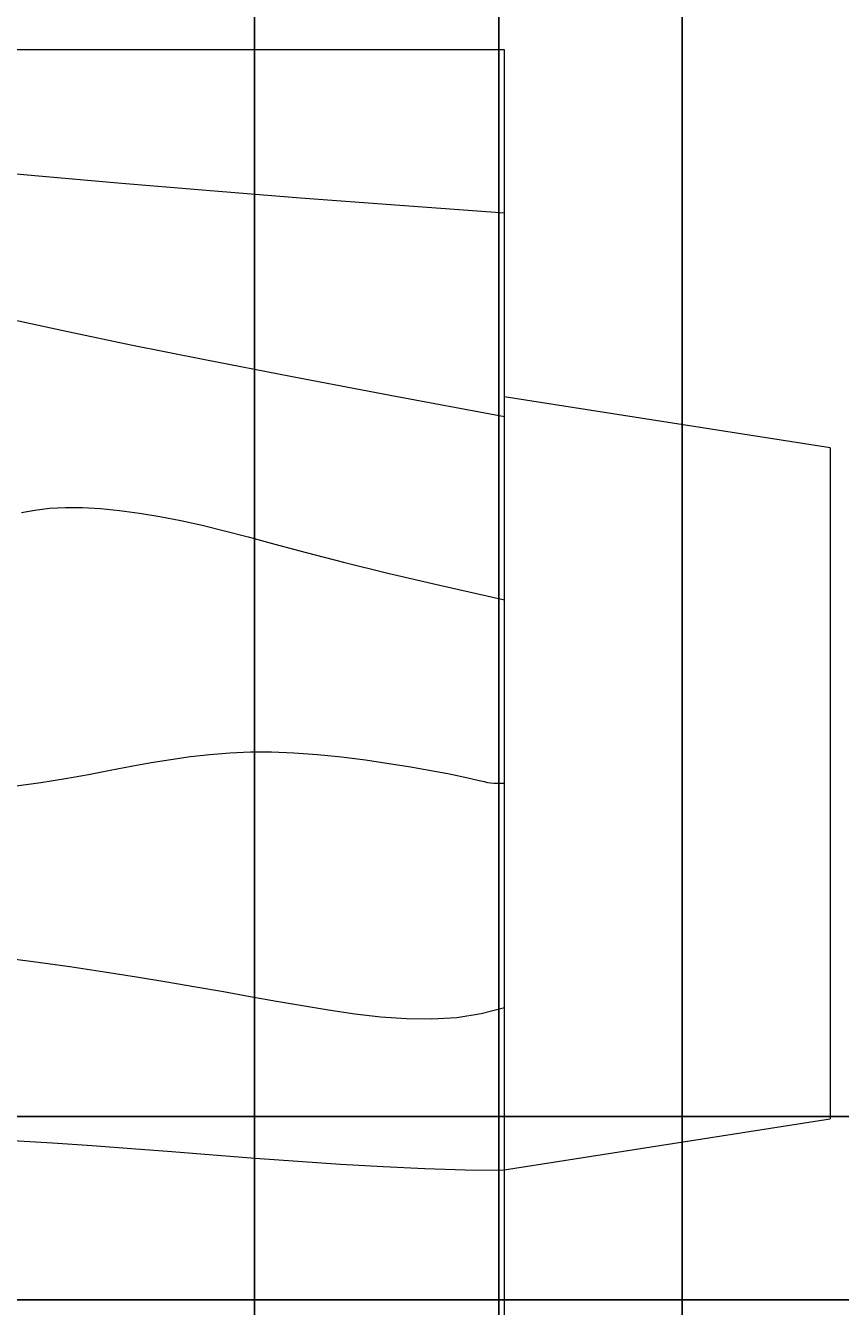
# Model space of a CAD drawing. Units: inches. Extents: x 7359 to 7979, y 33027 to 34263.
# Tile 11 of 32: x 7728 to 7748, y 33386 to 33417. Entities that reach past the tile are written whole.
import ezdxf

# ---------------------------------------------------------------- set-up
doc = ezdxf.new("R2010")
doc.units = ezdxf.units.IN
doc.layers.add('A-ANNO-DIMS', color=2, linetype='Continuous', lineweight=18)
doc.layers.add('A-FURN', color=8, linetype='Continuous', lineweight=18)
doc.styles.get("Standard").update_dxf_attribs({"font": 'arial.ttf'})
doc.dimstyles.get("Standard").update_dxf_attribs({"dimtxt": 0.18, "dimasz": 0.18, "dimexe": 0.18, "dimexo": 0.0625, "dimgap": 0.09, "dimtad": 0, "dimtih": 1, "dimtoh": 1, "dimdec": 4, "dimzin": 0, "dimdsep": 46, "dimtxsty": 'Standard', "dimcen": 0.09, "dimadec": 0, "dimazin": 0, "dimtfac": 1, "dimtdec": 4, "dimtofl": 0, "dimtmove": 0, "dimatfit": 3, "dimfxl": 1, "dimtolj": 1, "dimtzin": 0, "dimarcsym": 0})

# ---------------------------------------------------------------- blocks, each defined once
blk = doc.blocks.new('Dining Set - 36 x 72 in.')
for p, q in [((36, 18), (-36, 18)), ((36, -18), (36, 18)), ((44.0006, 8.23428), (35.9976, 9.48474)), ((44, 8.23041), (44, -8.23915)), ((35.9976, -9.48476), (43.9993, -8.2345))]:
    blk.add_line(p, q)
for points in [[(22.5879, 15.08984), (24.4721, 14.91715), (26.5052, 14.73958), (28.6809, 14.5581), (30.9929, 14.3737), (33.4347, 14.18733), (36, 14)], [(23.959, 11.37304), (25.2786, 11.08618), (26.8282, 10.76562), (28.6414, 10.40405), (30.752, 9.99414), (33.1936, 9.52856), (36, 9)], [(24.142, 6.64323), (24.4735, 6.70735), (24.8334, 6.75), (25.2235, 6.76969), (25.642, 6.76692), (26.0858, 6.74267), (26.5521, 6.69791), (27.0379, 6.63362), (27.5404, 6.55078), (28.0565, 6.45036), (28.5834, 6.33333), (29.1242, 6.19987), (29.7071, 6.04687), (30.3661, 5.87044), (31.1354, 5.66666), (32.0493, 5.43164), (33.142, 5.16146), (34.4475, 4.85221), (36, 4.5)], [(23.9549, -0.06836), (24.6146, 0.02083), (25.2235, 0.11784), (25.7904, 0.21875), (26.3241, 0.31966), (26.8334, 0.41666), (27.3265, 0.50618), (27.8099, 0.58593), (28.2894, 0.65397), (28.7709, 0.70833), (29.2601, 0.74707), (29.763, 0.76823), (30.2855, 0.76985), (30.8334, 0.75), (31.4088, 0.70784), (31.9994, 0.64713), (32.589, 0.57275), (33.1615, 0.48958), (33.7008, 0.4025), (34.1908, 0.3164), (34.6153, 0.23616), (34.9584, 0.16666), (35.2099, 0.11165), (35.3848, 0.07031), (35.504, 0.04069), (35.5886, 0.02083), (35.6594, 0.00879), (35.7377, 0.0026), (35.8442, 0.00032), (36, 0)], [(23.4727, -4.25391), (24.4289, -4.37549), (25.3334, -4.5), (26.1785, -4.62492), (26.9694, -4.74935), (27.7145, -4.87281), (28.4219, -4.99479), (29.1, -5.11483), (29.7572, -5.23242), (30.4016, -5.34709), (31.0417, -5.45834), (31.6837, -5.56437), (32.3262, -5.65821), (32.9658, -5.73153), (33.599, -5.77604), (34.2224, -5.78345), (34.8327, -5.74545), (35.4264, -5.65373), (36, -5.5)], [(23.9271, -8.76563), (24.9081, -8.82707), (25.8763, -8.89388), (26.8465, -8.96558), (27.8334, -9.04167), (28.8474, -9.12118), (29.8828, -9.20117), (30.93, -9.27824), (31.9792, -9.34896), (33.0205, -9.40991), (34.0443, -9.45768), (35.0407, -9.48885), (36, -9.5)]]:
    blk.add_lwpolyline(points)
blk = doc.blocks.new('*D74')
at = {"layer": 'A-ANNO-DIMS', "color": 0, "lineweight": -2, "transparency": 16777216}
for p, q in [((7743.727, 33618.1), (7743.727, 33027.177)), ((7787.034, 33618.1), (7787.034, 33027.177)), ((7743.907, 33027.357), (7765, 33027.357)), ((7786.854, 33027.357), (7765.76, 33027.357))]:
    blk.add_line(p, q, dxfattribs=at)
at = {"layer": 'A-ANNO-DIMS', "color": 0, "transparency": 16777216}
for points in [[(7743.907, 33027.387), (7743.907, 33027.327), (7743.727, 33027.357)], [(7786.854, 33027.387), (7786.854, 33027.327), (7787.034, 33027.357)]]:
    blk.add_solid(points, dxfattribs=at)
at = {"layer": 'Defpoints', "color": 0, "transparency": 16777216}
for p in [(7743.727, 33618.162), (7787.034, 33618.162), (7787.034, 33027.357)]:
    blk.add_point(p, dxfattribs=at)
at = {"layer": 'A-ANNO-DIMS', "color": 0, "transparency": 16777216, "insert": (7765.38, 33027.357), "char_height": 0.18, "attachment_point": 5}
blk.add_mtext('\\A1;43.31', dxfattribs=at)
blk = doc.blocks.new('*D85')
at = {"layer": 'A-ANNO-DIMS', "color": 0, "lineweight": -2, "transparency": 16777216}
for p, q in [((7793.064, 33390.662), (7369.542, 33390.662)), ((7369.722, 33390.482), (7369.722, 33388.594)), ((7369.722, 33386.342), (7369.722, 33388.231)), ((7793.064, 33386.162), (7369.542, 33386.162))]:
    blk.add_line(p, q, dxfattribs=at)
at = {"layer": 'A-ANNO-DIMS', "color": 0, "transparency": 16777216}
for points in [[(7369.692, 33390.482), (7369.752, 33390.482), (7369.722, 33390.662)], [(7369.692, 33386.342), (7369.752, 33386.342), (7369.722, 33386.162)]]:
    blk.add_solid(points, dxfattribs=at)
at = {"layer": 'Defpoints', "color": 0, "transparency": 16777216}
for p in [(7793.127, 33390.662), (7369.722, 33386.162), (7793.127, 33386.162)]:
    blk.add_point(p, dxfattribs=at)
at = {"layer": 'A-ANNO-DIMS', "color": 0, "transparency": 16777216, "insert": (7369.722, 33388.412), "char_height": 0.18, "attachment_point": 5}
blk.add_mtext('\\A1;4.5', dxfattribs=at)
blk = doc.blocks.new('*D86')
at = {"layer": 'A-ANNO-DIMS', "color": 0, "lineweight": -2, "transparency": 16777216}
for p, q in [((7733.226578, 33475.599789), (7733.226578, 33027.176807)), ((7739.226578, 33475.599789), (7739.226578, 33027.176807)), ((7733.406578, 33027.356807), (7736.077151, 33027.356807)), ((7739.046578, 33027.356807), (7736.376005, 33027.356807))]:
    blk.add_line(p, q, dxfattribs=at)
at = {"layer": 'A-ANNO-DIMS', "color": 0, "transparency": 16777216}
for points in [[(7733.406578, 33027.386807), (7733.406578, 33027.326807), (7733.226578, 33027.356807)], [(7739.046578, 33027.386807), (7739.046578, 33027.326807), (7739.226578, 33027.356807)]]:
    blk.add_solid(points, dxfattribs=at)
at = {"layer": 'Defpoints', "color": 0, "transparency": 16777216}
for p in [(7733.226578, 33475.662289), (7739.226578, 33475.662289), (7739.226578, 33027.356807)]:
    blk.add_point(p, dxfattribs=at)
at = {"layer": 'A-ANNO-DIMS', "color": 0, "transparency": 16777216, "insert": (7736.226578, 33027.356807), "char_height": 0.18, "attachment_point": 5}
blk.add_mtext('\\A1;6', dxfattribs=at)
blk = doc.blocks.new('*D87')
at = {"layer": 'A-ANNO-DIMS', "color": 0, "lineweight": -2, "transparency": 16777216}
for p, q in [((7743.726578, 33453.099789), (7743.726578, 33027.176807)), ((7749.726578, 33453.099789), (7749.726578, 33027.176807)), ((7743.906578, 33027.356807), (7746.577151, 33027.356807)), ((7749.546578, 33027.356807), (7746.876005, 33027.356807))]:
    blk.add_line(p, q, dxfattribs=at)
at = {"layer": 'A-ANNO-DIMS', "color": 0, "transparency": 16777216}
for points in [[(7743.906578, 33027.386807), (7743.906578, 33027.326807), (7743.726578, 33027.356807)], [(7749.546578, 33027.386807), (7749.546578, 33027.326807), (7749.726578, 33027.356807)]]:
    blk.add_solid(points, dxfattribs=at)
at = {"layer": 'Defpoints', "color": 0, "transparency": 16777216}
for p in [(7743.726578, 33453.162289), (7749.726578, 33453.162289), (7749.726578, 33027.356807)]:
    blk.add_point(p, dxfattribs=at)
at = {"layer": 'A-ANNO-DIMS', "color": 0, "transparency": 16777216, "insert": (7746.726578, 33027.356807), "char_height": 0.18, "attachment_point": 5}
blk.add_mtext('\\A1;6', dxfattribs=at)

msp = doc.modelspace()

# ---------------------------------------------------------------- block references
at = {"layer": 'A-FURN'}
msp.add_blockref('Dining Set - 36 x 72 in.', (7703.363, 33398.8436), dxfattribs=at)

# ---------------------------------------------------------------- dimensions: what is measured, and where the dimension line sits
at = {"layer": 'A-ANNO-DIMS'}
for base, p1, p2, override, picture, middle in [((7787.0342, 33027.3568), (7743.7266, 33618.1623), (7787.0342, 33618.1623), {"dimdec": 2, "dimlfac": 1, "dimrnd": 0, "dimzin": 0, "dimdsep": 46, "dimlunit": 2}, '*D74', (7765.3804, 33027.3568)), ((7739.2266, 33027.3568), (7733.2266, 33475.6623), (7739.2266, 33475.6623), {"dimdec": 0, "dimlfac": 1, "dimrnd": 0, "dimzin": 0, "dimdsep": 46, "dimlunit": 2}, '*D86', (7736.2266, 33027.3568)), ((7749.7266, 33027.3568), (7743.7266, 33453.1623), (7749.7266, 33453.1623), {"dimdec": 0, "dimlfac": 1, "dimrnd": 0, "dimzin": 0, "dimdsep": 46, "dimlunit": 2}, '*D87', (7746.7266, 33027.3568))]:
    dim = msp.add_linear_dim(base=base, p1=p1, p2=p2, dimstyle='Standard', override=override, dxfattribs=at)
    dim.commit()
    dim.dimension.update_dxf_attribs({"geometry": picture, "text_midpoint": middle})
dim = msp.add_linear_dim(base=(7369.7217, 33386.1623), p1=(7793.1266, 33390.6623), p2=(7793.1266, 33386.1623), angle=90, dimstyle='Standard', override={"dimdec": 1, "dimlfac": 1, "dimrnd": 0, "dimzin": 0, "dimdsep": 46, "dimlunit": 2}, dxfattribs=at)
dim.commit()
dim.dimension.update_dxf_attribs({"geometry": '*D85', "text_midpoint": (7369.7217, 33388.4123)})

doc.saveas('drawing.dxf')
